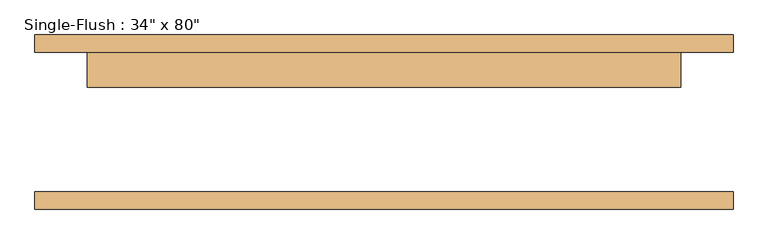
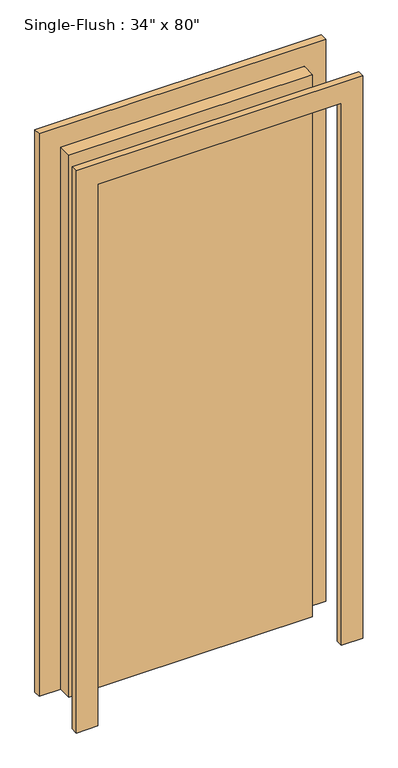
"""IFC4 building model written with IfcOpenShell, lengths in millimetres: door geometry."""

from ifc_helpers import new_model, si_unit, frame, origin, origin_with_axes, place, context, project, spatial, polyline, outline, extrude, source, transform, mapped, element, save


def door_ef9e9df2(model_context):
    return source(origin(), model_context, "Body", "SweptSolid", [
        extrude(outline(polyline([(2108.2, -508.0), (0.0, -508.0), (0.0, -431.8), (2032.0, -431.8), (2032.0, 431.8), (0.0, 431.8), (0.0, 508.0), (2108.2, 508.0), (2108.2, -508.0)])), frame((0.0, 101.6, 0.0), z_axis=(0.0, 1.0, 0.0), x_axis=(0.0, 0.0, 1.0)), (0.0, 0.0, 1.0), 25.4),
        extrude(outline(polyline([(2108.2, 508.0), (2108.2, -508.0), (0.0, -508.0), (0.0, -431.8), (2032.0, -431.8), (2032.0, 431.8), (0.0, 431.8), (0.0, 508.0), (2108.2, 508.0)])), frame((0.0, -127.0, 0.0), z_axis=(0.0, 1.0, 0.0), x_axis=(0.0, 0.0, 1.0)), (0.0, 0.0, 1.0), 25.4),
        extrude(outline(polyline([(431.8, 50.8), (-431.8, 50.8), (-431.8, 101.6), (431.8, 101.6), (431.8, 50.8)])), origin_with_axes(), (0.0, 0.0, 1.0), 2032.0),
    ])


if __name__ == "__main__":
    model = new_model("IFC4")
    model_context = context("Model", 3, world=origin())
    ifc_project = project(units=[si_unit("LENGTHUNIT", "METRE", prefix="MILLI")], contexts=[model_context])
    site = spatial("IfcSite", under=ifc_project)
    building = spatial("IfcBuilding", under=site)
    placement = place(None, origin())
    door_shape = door_ef9e9df2(model_context)
    element("IfcDoor", 1, ObjectType="Single-Flush : 34\" x 80\"", at=placement, inside=building, context=model_context, shape_type="MappedRepresentation", body=[
        mapped(door_shape, transform((0.0, 0.0, 0.0), x_axis=(1.0, 0.0, 0.0), y_axis=(0.0, 1.0, 0.0), z_axis=(0.0, 0.0, 1.0))),
    ])
    save(model, "model.ifc")

# Revit data of these elements
# Type "Single-Flush : 34\" x 80\""
#   Type Mark = "7"
#   Construction Type Id = "MDOOR"
#   Assembly Code = "C1020"
#   Analytic Construction = "Metal"
#   Thickness = 0' - 2"
#   Heat Transfer Coefficient (U) = 0.651978 BTU/(h·ft²·°F)
#   Height = 6' - 8"
#   Trim Projection Ext = 0' - 1"
#   Trim Projection Int = 0' - 1"
#   Trim Width = 0' - 3"
#   Width = 2' - 10"
#   Define Thermal Properties by = 1
#   Door Material = Door - Panel
#   Frame Material = Door - Frame
#   Visual Light Transmittance = 0
#   Solar Heat Gain Coefficient = 0
#   Function = (empty or 0)
#   Wall Closure = (empty or 0)
# Element 1 (IfcDoor, "Single-Flush : 34\" x 80\"")
#   Materials on its faces: "Door - Frame", "Door - Panel"
# Materials
#   "Door - Panel": class "Wood", colour RGB 210 159 95, transparency 0
#   "Door - Frame": colour RGB 118 70 51, transparency 0
